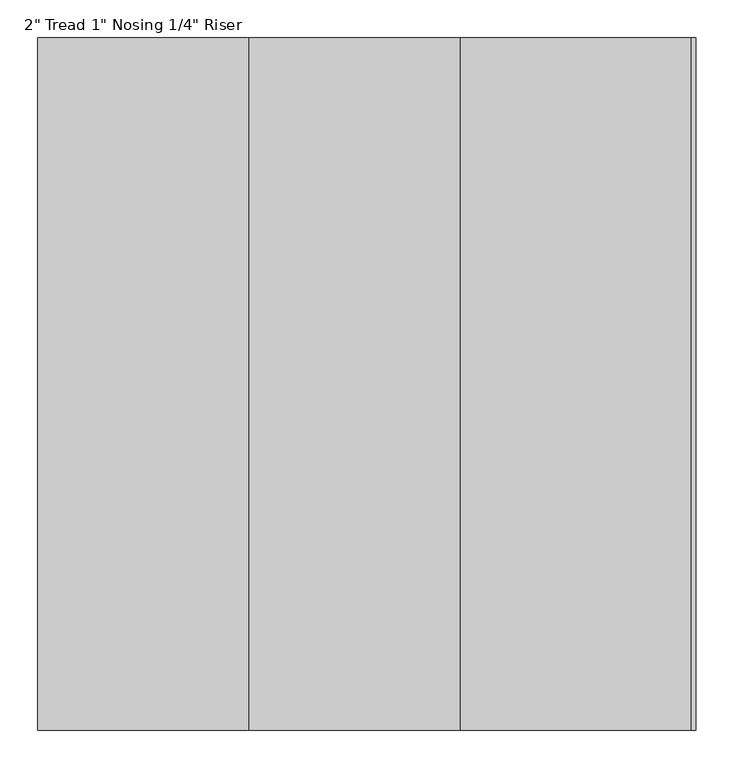
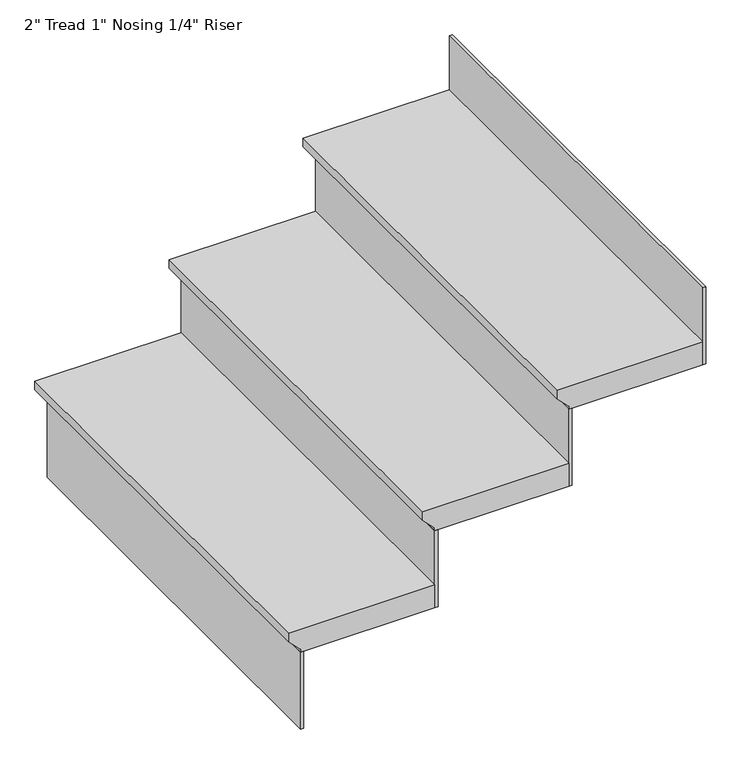
"""IFC4 building model written with IfcOpenShell, lengths in millimetres: stair flight geometry."""

from ifc_helpers import new_model, si_unit, frame, origin, place, context, project, spatial, polyline, outline, extrude, source, transform, mapped, element, save


def stair_flight_a2e4d9b1(model_context):
    return source(origin(), model_context, "Body", "SweptSolid", [
        extrude(outline(polyline([(2506.1333333, -9769.5522729), (2506.1333333, -10074.3522729), (2487.0833333, -10074.3522729), (2461.6833333, -10048.9522729), (2455.3333333, -10048.9522729), (2455.3333333, -9769.5522729), (2506.1333333, -9769.5522729)])), frame((0.0, -2916.0844117, 0.0), z_axis=(0.0, 1.0, 0.0), x_axis=(0.0, 0.0, 1.0)), (0.0, 0.0, 1.0), 914.4),
        extrude(outline(polyline([(-10042.6022729, -2916.0844117), (-10048.9522729, -2916.0844117), (-10048.9522729, -2001.6844117), (-10042.6022729, -2001.6844117), (-10042.6022729, -2916.0844117)])), frame((0.0, 0.0, 2286.0), z_axis=(0.0, 0.0, 1.0), x_axis=(1.0, 0.0, 0.0)), (0.0, 0.0, 1.0), 169.3333333),
        extrude(outline(polyline([(-9763.2022729, -2916.0844117), (-9769.5522729, -2916.0844117), (-9769.5522729, -2001.6844117), (-9763.2022729, -2001.6844117), (-9763.2022729, -2916.0844117)])), frame((0.0, 0.0, 2455.3333333), z_axis=(0.0, 0.0, 1.0), x_axis=(1.0, 0.0, 0.0)), (0.0, 0.0, 1.0), 169.3333333),
        extrude(outline(polyline([(2675.4666667, -9490.1522729), (2675.4666667, -9794.9522729), (2656.4166667, -9794.9522729), (2631.0166667, -9769.5522729), (2624.6666667, -9769.5522729), (2624.6666667, -9490.1522729), (2675.4666667, -9490.1522729)])), frame((0.0, -2916.0844117, 0.0), z_axis=(0.0, 1.0, 0.0), x_axis=(0.0, 0.0, 1.0)), (0.0, 0.0, 1.0), 914.4),
        extrude(outline(polyline([(-9483.8022729, -2916.0844117), (-9490.1522729, -2916.0844117), (-9490.1522729, -2001.6844117), (-9483.8022729, -2001.6844117), (-9483.8022729, -2916.0844117)])), frame((0.0, 0.0, 2624.6666667), z_axis=(0.0, 0.0, 1.0), x_axis=(1.0, 0.0, 0.0)), (0.0, 0.0, 1.0), 169.3333333),
        extrude(outline(polyline([(-9204.4022729, -2916.0844117), (-9210.7522729, -2916.0844117), (-9210.7522729, -2001.6844117), (-9204.4022729, -2001.6844117), (-9204.4022729, -2916.0844117)])), frame((0.0, 0.0, 2794.0), z_axis=(0.0, 0.0, 1.0), x_axis=(1.0, 0.0, 0.0)), (0.0, 0.0, 1.0), 169.3333333),
        extrude(outline(polyline([(2844.8, -9210.7522729), (2844.8, -9515.5522729), (2825.75, -9515.5522729), (2800.35, -9490.1522729), (2794.0, -9490.1522729), (2794.0, -9210.7522729), (2844.8, -9210.7522729)])), frame((0.0, -2916.0844117, 0.0), z_axis=(0.0, 1.0, 0.0), x_axis=(0.0, 0.0, 1.0)), (0.0, 0.0, 1.0), 914.4),
    ])


if __name__ == "__main__":
    model = new_model("IFC4")
    model_context = context("Model", 3, world=origin())
    ifc_project = project(units=[si_unit("LENGTHUNIT", "METRE", prefix="MILLI")], contexts=[model_context])
    site = spatial("IfcSite", under=ifc_project)
    building = spatial("IfcBuilding", under=site)
    placement = place(None, origin())
    stair_flight_shape = stair_flight_a2e4d9b1(model_context)
    element("IfcStairFlight", 1, ObjectType="2\" Tread 1\" Nosing 1/4\" Riser", at=placement, inside=building, context=model_context, shape_type="MappedRepresentation", body=[
        mapped(stair_flight_shape, transform((0.0, 0.0, 0.0), x_axis=(1.0, 0.0, 0.0), y_axis=(0.0, 1.0, 0.0), z_axis=(0.0, 0.0, 1.0))),
    ])
    save(model, "model.ifc")
